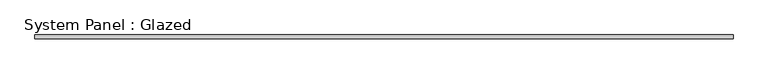
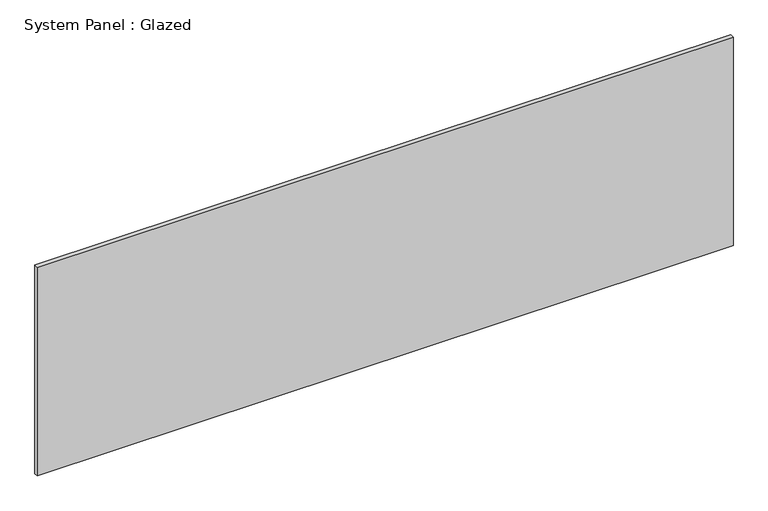
"""IFC4 building model written with IfcOpenShell, lengths in millimetres: plate geometry, System Panel : Glazed."""

from ifc_helpers import new_model, si_unit, origin, origin_with_axes, place, context, project, spatial, polyline, outline, extrude, source, transform, mapped, element, save


def system_panel_glazed_627c678d(model_context):
    return source(origin(), model_context, "Body", "SweptSolid", [
        extrude(outline(polyline([(2302.5628111, 19.05), (-2302.5628111, 19.05), (-2302.5628111, 44.45), (2302.5628111, 44.45), (2302.5628111, 19.05)])), origin_with_axes(), (0.0, 0.0, 1.0), 1460.5),
    ])


if __name__ == "__main__":
    model = new_model("IFC4")
    model_context = context("Model", 3, world=origin())
    ifc_project = project(units=[si_unit("LENGTHUNIT", "METRE", prefix="MILLI")], contexts=[model_context])
    site = spatial("IfcSite", under=ifc_project)
    building = spatial("IfcBuilding", under=site)
    placement = place(None, origin())
    system_panel_glazed_shape = system_panel_glazed_627c678d(model_context)
    element("IfcPlate", 1, ObjectType="System Panel : Glazed", at=placement, inside=building, context=model_context, shape_type="MappedRepresentation", body=[
        mapped(system_panel_glazed_shape, transform((0.0, 0.0, 0.0), x_axis=(1.0, 0.0, 0.0), y_axis=(0.0, 1.0, 0.0), z_axis=(0.0, 0.0, 1.0))),
    ])
    save(model, "model.ifc")

# Revit data of these elements
# Type "System Panel : Glazed"
#   Construction Type Id = "GSP4R"
#   Analytic Construction = "1/8 in Pilkington single glazing"
#   Visual Light Transmittance = 0.9
#   Solar Heat Gain Coefficient = 0.86
#   Heat Transfer Coefficient (U) = 1.18115 BTU/(h·ft²·°F)
# Element 1 (IfcPlate, "System Panel : Glazed")
#   Materials on its faces: "Glass"
# Materials
#   "Glass": class "Glass", colour RGB 0 128 192, transparency 0.75, Description = "Soda Lime Glass", Cost = 0
